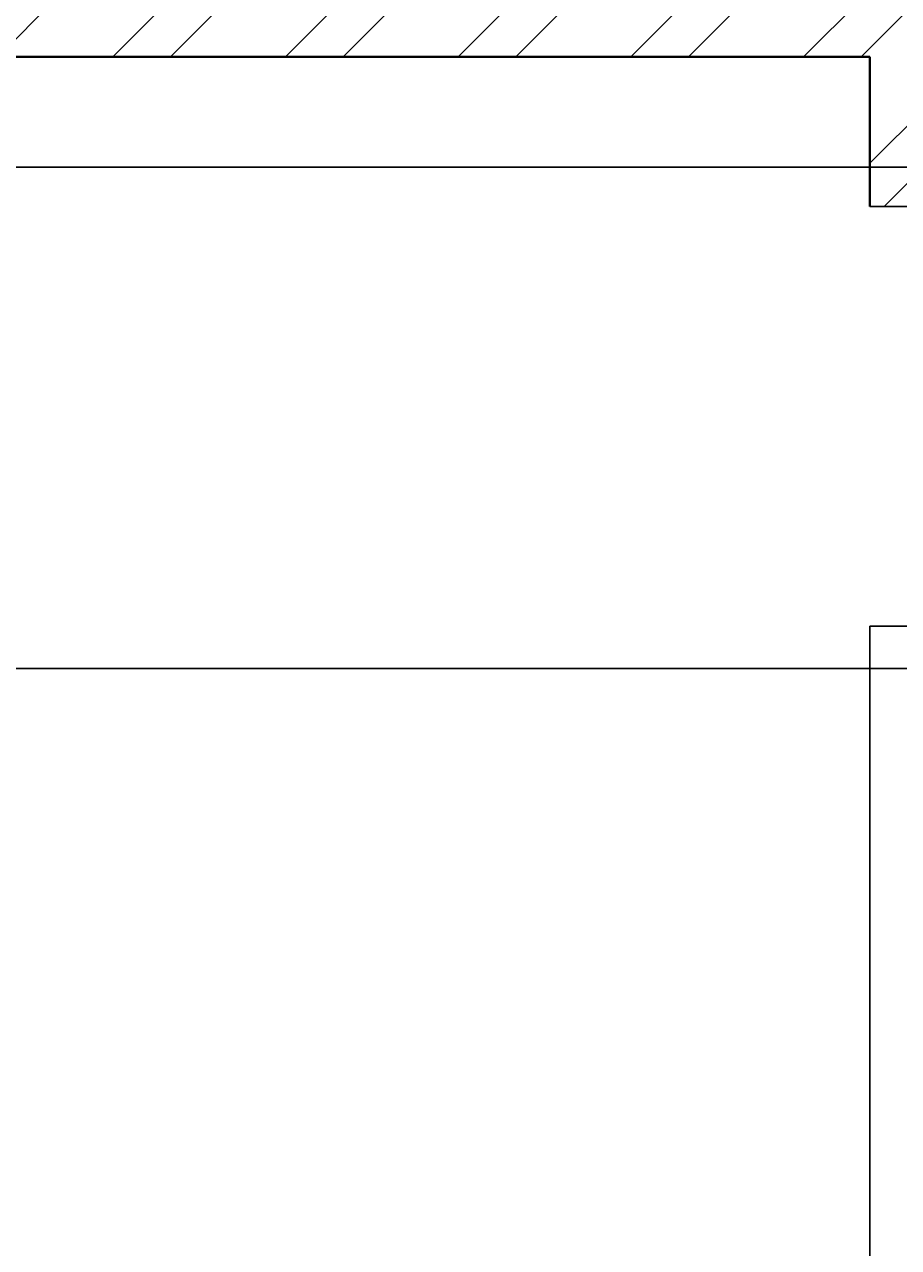
# Model space of a CAD drawing. Units: inches. Extents: x 1601 to 2297, y 1496 to 2631.
# Tile 54 of 57: x 2103 to 2171, y 2327 to 2422. Entities that reach past the tile are written whole.
import ezdxf

# ---------------------------------------------------------------- set-up
doc = ezdxf.new("R2010")
doc.units = ezdxf.units.IN
for name, color, linetype, lineweight in [('A-ANNO-DIMS', 2, 'Continuous', 18), ('A-DOOR', 21, 'Continuous', 25), ('A-WALL', 7, 'Continuous', 40), ('A-WALL-PATT', 215, 'Continuous', 13)]:
    doc.layers.add(name, color=color, linetype=linetype, lineweight=lineweight)
doc.styles.get("Standard").update_dxf_attribs({"font": 'arial.ttf'})
doc.dimstyles.get("Standard").update_dxf_attribs({"dimtxt": 0.18, "dimasz": 0.18, "dimexe": 0.18, "dimexo": 0.0625, "dimgap": 0.09, "dimtad": 0, "dimtih": 1, "dimtoh": 1, "dimdec": 4, "dimzin": 0, "dimdsep": 46, "dimtxsty": 'Standard', "dimcen": 0.09, "dimadec": 0, "dimazin": 0, "dimtfac": 1, "dimtdec": 4, "dimtofl": 0, "dimtmove": 0, "dimatfit": 3, "dimfxl": 1, "dimtolj": 1, "dimtzin": 0, "dimarcsym": 0})

# ---------------------------------------------------------------- blocks, each defined once
blk = doc.blocks.new('*D51')
at = {"layer": 'A-ANNO-DIMS', "color": 0, "lineweight": -2, "transparency": 16777216}
for p, q in [((1912.152, 2411.194), (2279.267, 2411.194)), ((2279.087, 2411.014), (2279.087, 2391.827)), ((2279.087, 2372.275), (2279.087, 2391.463)), ((1912.152, 2372.095), (2279.267, 2372.095))]:
    blk.add_line(p, q, dxfattribs=at)
at = {"layer": 'A-ANNO-DIMS', "color": 0, "transparency": 16777216}
for points in [[(2279.057, 2411.014), (2279.117, 2411.014), (2279.087, 2411.194)], [(2279.057, 2372.275), (2279.117, 2372.275), (2279.087, 2372.095)]]:
    blk.add_solid(points, dxfattribs=at)
at = {"layer": 'Defpoints', "color": 0, "transparency": 16777216}
for p in [(1912.09, 2411.194), (2279.087, 2411.194), (1912.09, 2372.095)]:
    blk.add_point(p, dxfattribs=at)
at = {"layer": 'A-ANNO-DIMS', "color": 0, "transparency": 16777216, "insert": (2279.087, 2391.645), "char_height": 0.18, "attachment_point": 5}
blk.add_mtext('\\A1;39.1', dxfattribs=at)

msp = doc.modelspace()

# ---------------------------------------------------------------- hatches: boundary and pattern name
at = {"layer": 'A-WALL-PATT'}
h = msp.add_hatch(dxfattribs=at)
h.set_pattern_fill('ANSI32', color=256)
h.paths.add_polyline_path([(2230.5373, 2532.3254), (2106.0595, 2532.3254), (2106.0595, 2523.3254), (2169.0373, 2523.3254), (2169.0373, 2424.3254), (2091.3989, 2424.3254), (2091.3989, 2419.8254), (2169.0373, 2419.8254), (2169.0373, 2408.1385), (2178.0373, 2408.1385), (2178.0373, 2419.8254), (2181.0581, 2419.8254), (2181.0581, 2422.0754), (2181.0581, 2424.3254), (2178.0373, 2424.3254), (2178.0373, 2523.3254), (2226.0373, 2523.3254), (2226.0373, 2424.3254), (2206.6251, 2424.3254), (2206.6251, 2419.8254), (2226.0373, 2419.8254), (2226.0373, 2299.8254), (2226.0373, 2295.3254), (2178.0373, 2295.3254), (2178.0373, 2312.1385), (2169.0373, 2312.1385), (2169.0373, 2295.3254), (2130.0373, 2295.3254), (2130.0373, 2279.1364), (2128.0593, 2279.1364), (2128.0593, 2274.6364), (2130.0373, 2274.6364), (2130.0373, 2260.7505), (2134.5373, 2260.7505), (2134.5373, 2290.8254), (2226.0373, 2290.8254), (2226.0373, 2279.2475), (2230.5373, 2279.2475), (2230.5373, 2347.8254)])
h.paths.add_polyline_path([(2070.0595, 2532.3254), (2031.0373, 2532.3254), (2031.0373, 2466.3254), (2003.9878, 2466.3254), (2003.9878, 2457.3254), (2031.0373, 2457.3254), (2031.0373, 2419.8254), (2031.0373, 2373.1914), (2035.5373, 2373.1914), (2035.5373, 2419.8254), (2047.3393, 2419.8254), (2047.3393, 2424.3254), (2035.5373, 2424.3254), (2035.5373, 2523.3254), (2070.0595, 2523.3254), (2070.0595, 2527.8254)])
h.paths.add_polyline_path([(1893.0373, 2532.3254), (1866.0336, 2532.3254), (1866.0336, 2523.3254), (1888.5373, 2523.3254), (1888.5373, 2347.8254), (1893.0373, 2347.8254), (1893.0373, 2457.3254), (1907.9878, 2457.3254), (1907.9878, 2466.3254), (1893.0373, 2466.3254)])

# ---------------------------------------------------------------- linework, layer by layer
at = {"layer": 'A-DOOR'}
for p, q in [((2169.0373, 2408.1385), (2178.0373, 2408.1385)), ((2169.0373, 2375.3908), (2169.0373, 2312.1385)), ((2169.0373, 2375.3908), (2173.5373, 2375.3908))]:
    msp.add_line(p, q, dxfattribs=at)
at = {"layer": 'A-WALL'}
for p, q in [((2091.3989, 2419.8254), (2169.0373, 2419.8254)), ((2169.0373, 2419.8254), (2169.0373, 2408.1385))]:
    msp.add_line(p, q, dxfattribs=at)

# ---------------------------------------------------------------- dimensions: what is measured, and where the dimension line sits
at = {"layer": 'A-ANNO-DIMS'}
dim = msp.add_linear_dim(base=(2279.0873, 2411.1939), p1=(1912.0896, 2372.0953), p2=(1912.0896, 2411.1939), angle=90, dimstyle='Standard', override={"dimdec": 1, "dimlfac": 1, "dimrnd": 0, "dimzin": 0, "dimdsep": 46, "dimlunit": 2}, dxfattribs=at)
dim.commit()
dim.dimension.update_dxf_attribs({"geometry": '*D51', "text_midpoint": (2279.0873, 2391.6446)})

doc.saveas('drawing.dxf')
